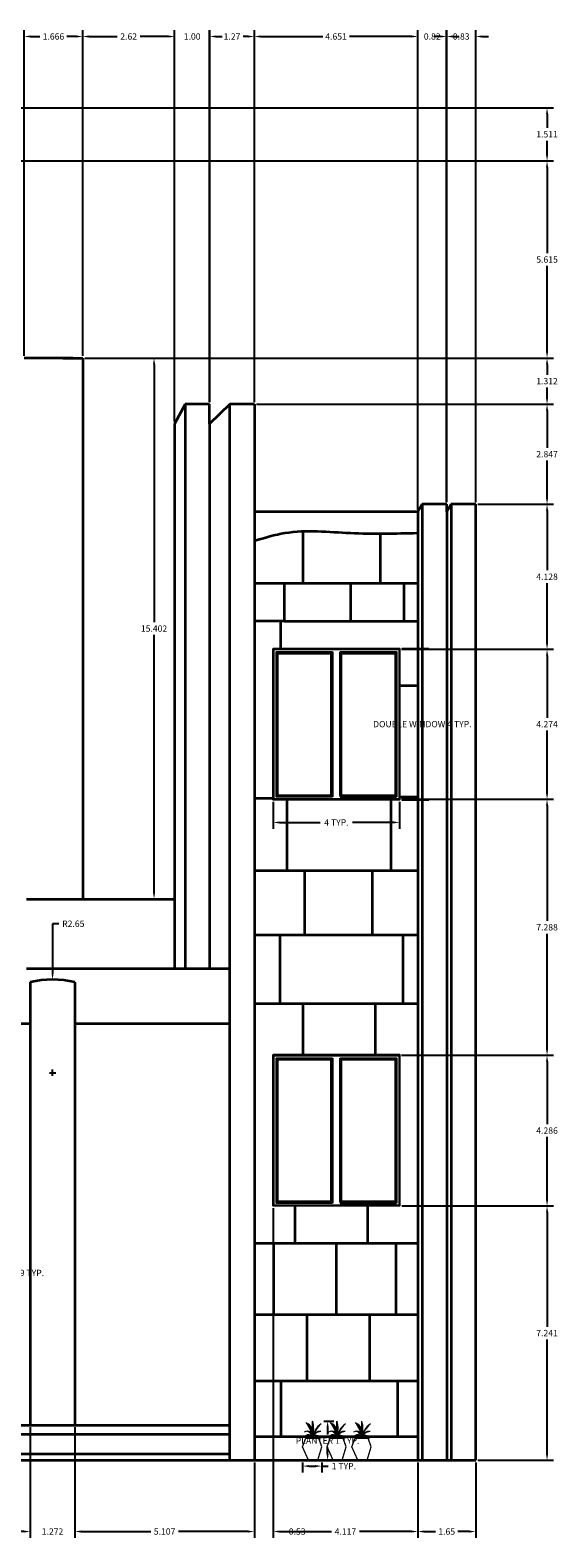
# Model space of a CAD drawing. Units: millimetres. Extents: x 2521.2 to 2565.9, y 755.2 to 798.1.
# Tile 3 of 3: x 2550.9 to 2565.9, y 755.2 to 798.1. Entities that reach past the tile are written whole.
import ezdxf

# ---------------------------------------------------------------- set-up
doc = ezdxf.new("R2010")
doc.units = ezdxf.units.MM
for name, color, linetype, lineweight in [('A-ANNO-DIMS', 2, 'Continuous', 18), ('A-ELEV', 7, 'Continuous', 35), ('A-GLAZ', 4, 'Continuous', 25), ('L-PLNT', 3, 'Continuous', 18)]:
    doc.layers.add(name, color=color, linetype=linetype, lineweight=lineweight)
doc.styles.get("Standard").update_dxf_attribs({"font": 'arial.ttf'})
doc.dimstyles.get("Standard").update_dxf_attribs({"dimtxt": 0.18, "dimasz": 0.18, "dimexe": 0.18, "dimexo": 0.0625, "dimgap": 0.09, "dimtad": 0, "dimtih": 1, "dimtoh": 1, "dimdec": 4, "dimzin": 0, "dimdsep": 46, "dimtxsty": 'Standard', "dimcen": 0.09, "dimadec": 0, "dimazin": 0, "dimtfac": 1, "dimtdec": 4, "dimtofl": 0, "dimtmove": 0, "dimatfit": 3, "dimfxl": 1, "dimtolj": 1, "dimtzin": 0, "dimarcsym": 0})

# ---------------------------------------------------------------- blocks, each defined once
blk = doc.blocks.new('WIN-DOUBLE')
for p, q in [((2559.456, 776.3), (2559.456, 780.343)), ((2559.491, 780.386), (2559.491, 776.258)), ((2559.716, 776.3), (2559.716, 780.386)), ((2559.756, 776.3), (2559.756, 780.343)), ((2559.716, 776.3), (2559.716, 776.258)), ((2559.716, 776.258), (2561.319, 776.258))]:
    blk.add_line(p, q)
for points in [[(2557.805, 780.483), (2561.406, 780.483), (2561.406, 776.176), (2557.805, 776.176)], [(2557.825, 780.462), (2561.393, 780.462), (2561.393, 776.189), (2557.825, 776.189)]]:
    blk.add_lwpolyline(points, close=True)
for points in [[(2559.491, 776.258), (2557.898, 776.258), (2557.898, 780.386), (2559.491, 780.386)], [(2559.456, 776.3), (2557.936, 776.3), (2557.936, 780.343), (2559.456, 780.343)], [(2559.716, 780.386), (2561.319, 780.386), (2561.319, 776.258)], [(2559.756, 780.343), (2561.276, 780.343), (2561.276, 776.3), (2559.756, 776.3)]]:
    blk.add_lwpolyline(points)
blk = doc.blocks.new('PLANTER')
for p, q in [((2558.646, 757.758), (2558.737, 758.005)), ((2558.817, 757.373), (2558.646, 757.758)), ((2558.737, 758.005), (2559.107, 758.005)), ((2559.08, 757.373), (2559.189, 757.758)), ((2559.189, 757.758), (2559.107, 758.005))]:
    blk.add_line(p, q)
for centre, radius, start, end in [((2558.164, 758.26), 0.796, 342.0282, 16.5628), ((2530.529, 758.527), 28.398, 358.9459, 359.9172), ((2558.772, 758.043), 0.155, 345.7039, 120.8927), ((2558.788, 757.931), 0.154, 28.8769, 113.7957), ((2558.504, 758.092), 0.427, 348.2161, 55.5831), ((2558.151, 757.944), 0.777, 5.6498, 40.0889), ((2558.161, 757.954), 0.763, 3.8104, 39.9888), ((2558.813, 757.985), 0.111, 10.1799, 119.9068), ((2558.697, 757.984), 0.226, 5.301, 71.0335), ((2558.66, 758.146), 0.293, 333.1798, 63.2065), ((2559.557, 757.89), 0.648, 126.493, 168.9551), ((2559.127, 757.986), 0.208, 79.6534, 172.2119), ((2559.023, 757.968), 0.112, 7.4318, 155.8017), ((2559.736, 757.784), 0.843, 132.0051, 164.8224), ((2559.176, 757.925), 0.266, 92.441, 162.4192), ((2559.033, 757.927), 0.136, 55.8779, 144.8755)]:
    blk.add_arc(centre, radius, start, end)
blk = doc.blocks.new('*D4')
at = {"layer": 'A-ANNO-DIMS', "color": 0, "lineweight": -2, "transparency": 16777216}
for p, q in [((2561.469, 780.483), (2562.232, 780.483)), ((2562.052, 780.303), (2562.052, 778.513)), ((2562.052, 776.356), (2562.052, 778.147)), ((2561.469, 776.176), (2562.232, 776.176))]:
    blk.add_line(p, q, dxfattribs=at)
at = {"layer": 'A-ANNO-DIMS', "color": 0, "transparency": 16777216}
for points in [[(2562.022, 780.303), (2562.082, 780.303), (2562.052, 780.483)], [(2562.022, 776.356), (2562.082, 776.356), (2562.052, 776.176)]]:
    blk.add_solid(points, dxfattribs=at)
at = {"layer": 'Defpoints', "color": 0, "transparency": 16777216}
for p in [(2561.406, 780.483), (2562.052, 780.483), (2561.406, 776.176)]:
    blk.add_point(p, dxfattribs=at)
at = {"layer": 'A-ANNO-DIMS', "color": 0, "transparency": 16777216, "insert": (2562.052, 778.33), "char_height": 0.18, "attachment_point": 5}
blk.add_mtext('\\A1;DOUBLE WINDOW 4 TYP.', dxfattribs=at)
blk = doc.blocks.new('*D5')
at = {"layer": 'A-ANNO-DIMS', "color": 0, "lineweight": -2, "transparency": 16777216}
for p, q in [((2557.805, 776.114), (2557.805, 775.35)), ((2561.406, 776.114), (2561.406, 775.35)), ((2557.985, 775.53), (2559.144, 775.53)), ((2561.226, 775.53), (2560.067, 775.53))]:
    blk.add_line(p, q, dxfattribs=at)
at = {"layer": 'A-ANNO-DIMS', "color": 0, "transparency": 16777216}
for points in [[(2557.985, 775.56), (2557.985, 775.5), (2557.805, 775.53)], [(2561.226, 775.56), (2561.226, 775.5), (2561.406, 775.53)]]:
    blk.add_solid(points, dxfattribs=at)
at = {"layer": 'Defpoints', "color": 0, "transparency": 16777216}
for p in [(2557.805, 776.176), (2561.406, 776.176), (2561.406, 775.53)]:
    blk.add_point(p, dxfattribs=at)
at = {"layer": 'A-ANNO-DIMS', "color": 0, "transparency": 16777216, "insert": (2559.606, 775.53), "char_height": 0.18, "attachment_point": 5}
blk.add_mtext('\\A1;4 TYP.', dxfattribs=at)
blk = doc.blocks.new('*D6')
at = {"layer": 'A-ANNO-DIMS', "color": 0, "lineweight": -2, "transparency": 16777216}
for p, q in [((2549.006, 767.037), (2550.423, 767.037)), ((2550.243, 766.857), (2550.243, 762.888)), ((2550.243, 758.553), (2550.243, 762.522)), ((2549.006, 758.373), (2550.423, 758.373))]:
    blk.add_line(p, q, dxfattribs=at)
at = {"layer": 'A-ANNO-DIMS', "color": 0, "transparency": 16777216}
for points in [[(2550.213, 766.857), (2550.273, 766.857), (2550.243, 767.037)], [(2550.213, 758.553), (2550.273, 758.553), (2550.243, 758.373)]]:
    blk.add_solid(points, dxfattribs=at)
at = {"layer": 'Defpoints', "color": 0, "transparency": 16777216}
for p in [(2548.944, 767.037), (2550.243, 767.037), (2548.944, 758.373)]:
    blk.add_point(p, dxfattribs=at)
at = {"layer": 'A-ANNO-DIMS', "color": 0, "transparency": 16777216, "insert": (2550.243, 762.705), "char_height": 0.18, "attachment_point": 5}
blk.add_mtext('\\A1;MAIN DOOR 9 TYP.', dxfattribs=at)
blk = doc.blocks.new('*D8')
at = {"layer": 'A-ANNO-DIMS', "color": 0, "lineweight": -2, "transparency": 16777216}
for p, q in [((2559.252, 758.486), (2559.536, 758.486)), ((2559.356, 758.306), (2559.356, 758.11)), ((2559.356, 757.553), (2559.356, 757.749)), ((2559.252, 757.373), (2559.536, 757.373))]:
    blk.add_line(p, q, dxfattribs=at)
at = {"layer": 'A-ANNO-DIMS', "color": 0, "transparency": 16777216}
for points in [[(2559.326, 758.306), (2559.386, 758.306), (2559.356, 758.486)], [(2559.326, 757.553), (2559.386, 757.553), (2559.356, 757.373)]]:
    blk.add_solid(points, dxfattribs=at)
at = {"layer": 'Defpoints', "color": 0, "transparency": 16777216}
for p in [(2559.189, 758.486), (2559.356, 758.486), (2559.189, 757.373)]:
    blk.add_point(p, dxfattribs=at)
at = {"layer": 'A-ANNO-DIMS', "color": 0, "transparency": 16777216, "insert": (2559.356, 757.93), "char_height": 0.18, "attachment_point": 5}
blk.add_mtext('\\A1;PLANTER 1 TYP.', dxfattribs=at)
blk = doc.blocks.new('*D9')
at = {"layer": 'A-ANNO-DIMS', "color": 0, "lineweight": -2, "transparency": 16777216}
for p, q in [((2558.646, 757.311), (2558.646, 757.026)), ((2558.826, 757.206), (2559.009, 757.206)), ((2559.189, 757.311), (2559.189, 757.026)), ((2559.189, 757.206), (2559.369, 757.206))]:
    blk.add_line(p, q, dxfattribs=at)
at = {"layer": 'A-ANNO-DIMS', "color": 0, "transparency": 16777216}
for points in [[(2558.826, 757.236), (2558.826, 757.176), (2558.646, 757.206)], [(2559.009, 757.236), (2559.009, 757.176), (2559.189, 757.206)]]:
    blk.add_solid(points, dxfattribs=at)
at = {"layer": 'Defpoints', "color": 0, "transparency": 16777216}
for p in [(2558.646, 757.373), (2559.189, 757.373), (2559.189, 757.206)]:
    blk.add_point(p, dxfattribs=at)
at = {"layer": 'A-ANNO-DIMS', "color": 0, "transparency": 16777216, "insert": (2559.819, 757.206), "char_height": 0.18, "attachment_point": 5}
blk.add_mtext('\\A1;1 TYP.', dxfattribs=at)
blk = doc.blocks.new('*D28')
at = {"layer": 'A-ANNO-DIMS', "color": 0, "lineweight": -2, "transparency": 16777216}
for p, q in [((2550.721, 788.812), (2550.721, 798.086)), ((2552.387, 788.812), (2552.387, 798.086)), ((2550.901, 797.906), (2551.169, 797.906)), ((2552.207, 797.906), (2551.939, 797.906))]:
    blk.add_line(p, q, dxfattribs=at)
at = {"layer": 'A-ANNO-DIMS', "color": 0, "transparency": 16777216}
for points in [[(2550.901, 797.936), (2550.901, 797.876), (2550.721, 797.906)], [(2552.207, 797.936), (2552.207, 797.876), (2552.387, 797.906)]]:
    blk.add_solid(points, dxfattribs=at)
at = {"layer": 'Defpoints', "color": 0, "transparency": 16777216}
for p in [(2552.387, 797.906), (2550.721, 788.75), (2552.387, 788.75)]:
    blk.add_point(p, dxfattribs=at)
at = {"layer": 'A-ANNO-DIMS', "color": 0, "transparency": 16777216, "insert": (2551.554, 797.906), "char_height": 0.18, "attachment_point": 5}
blk.add_mtext('\\A1;1.666', dxfattribs=at)
blk = doc.blocks.new('*D29')
at = {"layer": 'A-ANNO-DIMS', "color": 0, "lineweight": -2, "transparency": 16777216}
for p, q in [((2552.387, 788.812), (2552.387, 798.086)), ((2555.002, 786.941), (2555.002, 798.086)), ((2552.567, 797.906), (2553.37, 797.906)), ((2554.822, 797.906), (2554.019, 797.906))]:
    blk.add_line(p, q, dxfattribs=at)
at = {"layer": 'A-ANNO-DIMS', "color": 0, "transparency": 16777216}
for points in [[(2552.567, 797.936), (2552.567, 797.876), (2552.387, 797.906)], [(2554.822, 797.936), (2554.822, 797.876), (2555.002, 797.906)]]:
    blk.add_solid(points, dxfattribs=at)
at = {"layer": 'Defpoints', "color": 0, "transparency": 16777216}
for p in [(2555.002, 797.906), (2552.387, 788.75), (2555.002, 786.879)]:
    blk.add_point(p, dxfattribs=at)
at = {"layer": 'A-ANNO-DIMS', "color": 0, "transparency": 16777216, "insert": (2553.694, 797.906), "char_height": 0.18, "attachment_point": 5}
blk.add_mtext('\\A1;2.62', dxfattribs=at)
blk = doc.blocks.new('*D30')
at = {"layer": 'A-ANNO-DIMS', "color": 0, "lineweight": -2, "transparency": 16777216}
for p, q in [((2555.002138, 786.94116), (2555.002138, 798.086169)), ((2555.999594, 787.500222), (2555.999594, 798.086169)), ((2554.822138, 797.906169), (2554.642138, 797.906169)), ((2556.179594, 797.906169), (2556.359594, 797.906169))]:
    blk.add_line(p, q, dxfattribs=at)
at = {"layer": 'A-ANNO-DIMS', "color": 0, "transparency": 16777216}
for points in [[(2554.822138, 797.936169), (2554.822138, 797.876169), (2555.002138, 797.906169)], [(2556.179594, 797.936169), (2556.179594, 797.876169), (2555.999594, 797.906169)]]:
    blk.add_solid(points, dxfattribs=at)
at = {"layer": 'Defpoints', "color": 0, "transparency": 16777216}
for p in [(2555.999594, 797.906169), (2555.999594, 787.437722), (2555.002138, 786.87866)]:
    blk.add_point(p, dxfattribs=at)
at = {"layer": 'A-ANNO-DIMS', "color": 0, "transparency": 16777216, "insert": (2555.500866, 797.906169), "char_height": 0.18, "attachment_point": 5}
blk.add_mtext('\\A1;1.00', dxfattribs=at)
blk = doc.blocks.new('*D31')
at = {"layer": 'A-ANNO-DIMS', "color": 0, "lineweight": -2, "transparency": 16777216}
for p, q in [((2556, 787.5), (2556, 798.086)), ((2557.271, 787.5), (2557.271, 798.086)), ((2556.18, 797.906), (2556.32, 797.906)), ((2557.091, 797.906), (2556.951, 797.906))]:
    blk.add_line(p, q, dxfattribs=at)
at = {"layer": 'A-ANNO-DIMS', "color": 0, "transparency": 16777216}
for points in [[(2556.18, 797.936), (2556.18, 797.876), (2556, 797.906)], [(2557.091, 797.936), (2557.091, 797.876), (2557.271, 797.906)]]:
    blk.add_solid(points, dxfattribs=at)
at = {"layer": 'Defpoints', "color": 0, "transparency": 16777216}
for p in [(2557.271, 797.906), (2556, 787.438), (2557.271, 787.438)]:
    blk.add_point(p, dxfattribs=at)
at = {"layer": 'A-ANNO-DIMS', "color": 0, "transparency": 16777216, "insert": (2556.635, 797.906), "char_height": 0.18, "attachment_point": 5}
blk.add_mtext('\\A1;1.27', dxfattribs=at)
blk = doc.blocks.new('*D32')
at = {"layer": 'A-ANNO-DIMS', "color": 0, "lineweight": -2, "transparency": 16777216}
for p, q in [((2557.271, 787.5), (2557.271, 798.086)), ((2561.922, 784.436), (2561.922, 798.086)), ((2557.451, 797.906), (2559.217, 797.906)), ((2561.742, 797.906), (2559.976, 797.906))]:
    blk.add_line(p, q, dxfattribs=at)
at = {"layer": 'A-ANNO-DIMS', "color": 0, "transparency": 16777216}
for points in [[(2557.451, 797.936), (2557.451, 797.876), (2557.271, 797.906)], [(2561.742, 797.936), (2561.742, 797.876), (2561.922, 797.906)]]:
    blk.add_solid(points, dxfattribs=at)
at = {"layer": 'Defpoints', "color": 0, "transparency": 16777216}
for p in [(2561.922, 797.906), (2557.271, 787.438), (2561.922, 784.373)]:
    blk.add_point(p, dxfattribs=at)
at = {"layer": 'A-ANNO-DIMS', "color": 0, "transparency": 16777216, "insert": (2559.596, 797.906), "char_height": 0.18, "attachment_point": 5}
blk.add_mtext('\\A1;4.651', dxfattribs=at)
blk = doc.blocks.new('*D33')
at = {"layer": 'A-ANNO-DIMS', "color": 0, "lineweight": -2, "transparency": 16777216}
for p, q in [((2561.921891, 784.435917), (2561.921891, 798.086169)), ((2562.744309, 784.652956), (2562.744309, 798.086169)), ((2561.741891, 797.906169), (2561.561891, 797.906169)), ((2562.924309, 797.906169), (2563.104309, 797.906169))]:
    blk.add_line(p, q, dxfattribs=at)
at = {"layer": 'A-ANNO-DIMS', "color": 0, "transparency": 16777216}
for points in [[(2561.741891, 797.936169), (2561.741891, 797.876169), (2561.921891, 797.906169)], [(2562.924309, 797.936169), (2562.924309, 797.876169), (2562.744309, 797.906169)]]:
    blk.add_solid(points, dxfattribs=at)
at = {"layer": 'Defpoints', "color": 0, "transparency": 16777216}
for p in [(2562.744309, 797.906169), (2561.921891, 784.373417), (2562.744309, 784.590456)]:
    blk.add_point(p, dxfattribs=at)
at = {"layer": 'A-ANNO-DIMS', "color": 0, "transparency": 16777216, "insert": (2562.3331, 797.906169), "char_height": 0.18, "attachment_point": 5}
blk.add_mtext('\\A1;0.82', dxfattribs=at)
blk = doc.blocks.new('*D34')
at = {"layer": 'A-ANNO-DIMS', "color": 0, "lineweight": -2, "transparency": 16777216}
for p, q in [((2562.744, 784.653), (2562.744, 798.086)), ((2563.571, 784.653), (2563.571, 798.086)), ((2562.564, 797.906), (2562.384, 797.906)), ((2563.751, 797.906), (2563.931, 797.906))]:
    blk.add_line(p, q, dxfattribs=at)
at = {"layer": 'A-ANNO-DIMS', "color": 0, "transparency": 16777216}
for points in [[(2562.564, 797.936), (2562.564, 797.876), (2562.744, 797.906)], [(2563.751, 797.936), (2563.751, 797.876), (2563.571, 797.906)]]:
    blk.add_solid(points, dxfattribs=at)
at = {"layer": 'Defpoints', "color": 0, "transparency": 16777216}
for p in [(2563.571, 797.906), (2562.744, 784.59), (2563.571, 784.59)]:
    blk.add_point(p, dxfattribs=at)
at = {"layer": 'A-ANNO-DIMS', "color": 0, "transparency": 16777216, "insert": (2563.158, 797.906), "char_height": 0.18, "attachment_point": 5}
blk.add_mtext('\\A1;0.83', dxfattribs=at)
blk = doc.blocks.new('*D46')
at = {"layer": 'A-ANNO-DIMS', "color": 0, "lineweight": -2, "transparency": 16777216}
for p, q in [((2550.891519, 758.310917), (2550.891519, 755.163417)), ((2552.163561, 758.310917), (2552.163561, 755.163417)), ((2550.711519, 755.343417), (2550.531519, 755.343417)), ((2552.343561, 755.343417), (2552.523561, 755.343417))]:
    blk.add_line(p, q, dxfattribs=at)
at = {"layer": 'A-ANNO-DIMS', "color": 0, "transparency": 16777216}
for points in [[(2550.711519, 755.373417), (2550.711519, 755.313417), (2550.891519, 755.343417)], [(2552.343561, 755.373417), (2552.343561, 755.313417), (2552.163561, 755.343417)]]:
    blk.add_solid(points, dxfattribs=at)
at = {"layer": 'Defpoints', "color": 0, "transparency": 16777216}
for p in [(2550.891519, 758.373417), (2552.163561, 758.373417), (2552.163561, 755.343417)]:
    blk.add_point(p, dxfattribs=at)
at = {"layer": 'A-ANNO-DIMS', "color": 0, "transparency": 16777216, "insert": (2551.52754, 755.343417), "char_height": 0.18, "attachment_point": 5}
blk.add_mtext('\\A1;1.272', dxfattribs=at)
blk = doc.blocks.new('*D47')
at = {"layer": 'A-ANNO-DIMS', "color": 0, "lineweight": -2, "transparency": 16777216}
for p, q in [((2552.164, 758.311), (2552.164, 755.163)), ((2557.271, 757.311), (2557.271, 755.163)), ((2552.344, 755.343), (2554.324, 755.343)), ((2557.091, 755.343), (2555.111, 755.343))]:
    blk.add_line(p, q, dxfattribs=at)
at = {"layer": 'A-ANNO-DIMS', "color": 0, "transparency": 16777216}
for points in [[(2552.344, 755.373), (2552.344, 755.313), (2552.164, 755.343)], [(2557.091, 755.373), (2557.091, 755.313), (2557.271, 755.343)]]:
    blk.add_solid(points, dxfattribs=at)
at = {"layer": 'Defpoints', "color": 0, "transparency": 16777216}
for p in [(2552.164, 758.373), (2557.271, 757.373), (2557.271, 755.343)]:
    blk.add_point(p, dxfattribs=at)
at = {"layer": 'A-ANNO-DIMS', "color": 0, "transparency": 16777216, "insert": (2554.717, 755.343), "char_height": 0.18, "attachment_point": 5}
blk.add_mtext('\\A1;5.107', dxfattribs=at)
blk = doc.blocks.new('*D48')
at = {"layer": 'A-ANNO-DIMS', "color": 0, "lineweight": -2, "transparency": 16777216}
for p, q in [((2557.805, 764.552), (2557.805, 755.163)), ((2557.271, 757.311), (2557.271, 755.163)), ((2557.091, 755.343), (2556.911, 755.343)), ((2557.985, 755.343), (2558.165, 755.343))]:
    blk.add_line(p, q, dxfattribs=at)
at = {"layer": 'A-ANNO-DIMS', "color": 0, "transparency": 16777216}
for points in [[(2557.091, 755.373), (2557.091, 755.313), (2557.271, 755.343)], [(2557.985, 755.373), (2557.985, 755.313), (2557.805, 755.343)]]:
    blk.add_solid(points, dxfattribs=at)
at = {"layer": 'Defpoints', "color": 0, "transparency": 16777216}
for p in [(2557.805, 764.614), (2557.271, 757.373), (2557.805, 755.343)]:
    blk.add_point(p, dxfattribs=at)
at = {"layer": 'A-ANNO-DIMS', "color": 0, "transparency": 16777216, "insert": (2558.489, 755.343), "char_height": 0.18, "attachment_point": 5}
blk.add_mtext('\\A1;0.53', dxfattribs=at)
blk = doc.blocks.new('*D49')
at = {"layer": 'A-ANNO-DIMS', "color": 0, "lineweight": -2, "transparency": 16777216}
for p, q in [((2557.805, 764.552), (2557.805, 755.163)), ((2561.922, 757.311), (2561.922, 755.163)), ((2557.985, 755.343), (2559.466, 755.343)), ((2561.742, 755.343), (2560.261, 755.343))]:
    blk.add_line(p, q, dxfattribs=at)
at = {"layer": 'A-ANNO-DIMS', "color": 0, "transparency": 16777216}
for points in [[(2557.985, 755.373), (2557.985, 755.313), (2557.805, 755.343)], [(2561.742, 755.373), (2561.742, 755.313), (2561.922, 755.343)]]:
    blk.add_solid(points, dxfattribs=at)
at = {"layer": 'Defpoints', "color": 0, "transparency": 16777216}
for p in [(2557.805, 764.614), (2561.922, 757.373), (2561.922, 755.343)]:
    blk.add_point(p, dxfattribs=at)
at = {"layer": 'A-ANNO-DIMS', "color": 0, "transparency": 16777216, "insert": (2559.863, 755.343), "char_height": 0.18, "attachment_point": 5}
blk.add_mtext('\\A1;4.117', dxfattribs=at)
blk = doc.blocks.new('*D50')
at = {"layer": 'A-ANNO-DIMS', "color": 0, "lineweight": -2, "transparency": 16777216}
for p, q in [((2561.922, 757.311), (2561.922, 755.163)), ((2563.571, 757.311), (2563.571, 755.163)), ((2562.102, 755.343), (2562.43, 755.343)), ((2563.391, 755.343), (2563.062, 755.343))]:
    blk.add_line(p, q, dxfattribs=at)
at = {"layer": 'A-ANNO-DIMS', "color": 0, "transparency": 16777216}
for points in [[(2562.102, 755.373), (2562.102, 755.313), (2561.922, 755.343)], [(2563.391, 755.373), (2563.391, 755.313), (2563.571, 755.343)]]:
    blk.add_solid(points, dxfattribs=at)
at = {"layer": 'Defpoints', "color": 0, "transparency": 16777216}
for p in [(2561.922, 757.373), (2563.571, 757.373), (2563.571, 755.343)]:
    blk.add_point(p, dxfattribs=at)
at = {"layer": 'A-ANNO-DIMS', "color": 0, "transparency": 16777216, "insert": (2562.746, 755.343), "char_height": 0.18, "attachment_point": 5}
blk.add_mtext('\\A1;1.65', dxfattribs=at)
blk = doc.blocks.new('*D51')
at = {"layer": 'A-ANNO-DIMS', "color": 0, "lineweight": -2, "transparency": 16777216}
for p, q in [((2561.469, 764.614), (2565.781, 764.614)), ((2565.601, 764.434), (2565.601, 761.174)), ((2565.601, 757.553), (2565.601, 760.814)), ((2563.634, 757.373), (2565.781, 757.373))]:
    blk.add_line(p, q, dxfattribs=at)
at = {"layer": 'A-ANNO-DIMS', "color": 0, "transparency": 16777216}
for points in [[(2565.571, 764.434), (2565.631, 764.434), (2565.601, 764.614)], [(2565.571, 757.553), (2565.631, 757.553), (2565.601, 757.373)]]:
    blk.add_solid(points, dxfattribs=at)
at = {"layer": 'Defpoints', "color": 0, "transparency": 16777216}
for p in [(2561.406, 764.614), (2565.601, 764.614), (2563.571, 757.373)]:
    blk.add_point(p, dxfattribs=at)
at = {"layer": 'A-ANNO-DIMS', "color": 0, "transparency": 16777216, "insert": (2565.601, 760.994), "char_height": 0.18, "attachment_point": 5}
blk.add_mtext('\\A1;7.241', dxfattribs=at)
blk = doc.blocks.new('*D52')
at = {"layer": 'A-ANNO-DIMS', "color": 0, "lineweight": -2, "transparency": 16777216}
for p, q in [((2561.455, 768.901), (2565.781, 768.901)), ((2565.601, 768.721), (2565.601, 766.939)), ((2565.601, 764.794), (2565.601, 766.576)), ((2561.469, 764.614), (2565.781, 764.614))]:
    blk.add_line(p, q, dxfattribs=at)
at = {"layer": 'A-ANNO-DIMS', "color": 0, "transparency": 16777216}
for points in [[(2565.571, 768.721), (2565.631, 768.721), (2565.601, 768.901)], [(2565.571, 764.794), (2565.631, 764.794), (2565.601, 764.614)]]:
    blk.add_solid(points, dxfattribs=at)
at = {"layer": 'Defpoints', "color": 0, "transparency": 16777216}
for p in [(2561.393, 768.901), (2565.601, 768.901), (2561.406, 764.614)]:
    blk.add_point(p, dxfattribs=at)
at = {"layer": 'A-ANNO-DIMS', "color": 0, "transparency": 16777216, "insert": (2565.601, 766.758), "char_height": 0.18, "attachment_point": 5}
blk.add_mtext('\\A1;4.286', dxfattribs=at)
blk = doc.blocks.new('*D53')
at = {"layer": 'A-ANNO-DIMS', "color": 0, "lineweight": -2, "transparency": 16777216}
for p, q in [((2561.455, 776.189), (2565.781, 776.189)), ((2565.601, 776.009), (2565.601, 772.726)), ((2565.601, 769.081), (2565.601, 772.363)), ((2561.455, 768.901), (2565.781, 768.901))]:
    blk.add_line(p, q, dxfattribs=at)
at = {"layer": 'A-ANNO-DIMS', "color": 0, "transparency": 16777216}
for points in [[(2565.571, 776.009), (2565.631, 776.009), (2565.601, 776.189)], [(2565.571, 769.081), (2565.631, 769.081), (2565.601, 768.901)]]:
    blk.add_solid(points, dxfattribs=at)
at = {"layer": 'Defpoints', "color": 0, "transparency": 16777216}
for p in [(2561.393, 776.189), (2565.601, 776.189), (2561.393, 768.901)]:
    blk.add_point(p, dxfattribs=at)
at = {"layer": 'A-ANNO-DIMS', "color": 0, "transparency": 16777216, "insert": (2565.601, 772.545), "char_height": 0.18, "attachment_point": 5}
blk.add_mtext('\\A1;7.288', dxfattribs=at)
blk = doc.blocks.new('*D54')
at = {"layer": 'A-ANNO-DIMS', "color": 0, "lineweight": -2, "transparency": 16777216}
for p, q in [((2561.455, 780.462), (2565.781, 780.462)), ((2565.601, 780.282), (2565.601, 778.506)), ((2565.601, 776.369), (2565.601, 778.145)), ((2561.455, 776.189), (2565.781, 776.189))]:
    blk.add_line(p, q, dxfattribs=at)
at = {"layer": 'A-ANNO-DIMS', "color": 0, "transparency": 16777216}
for points in [[(2565.571, 780.282), (2565.631, 780.282), (2565.601, 780.462)], [(2565.571, 776.369), (2565.631, 776.369), (2565.601, 776.189)]]:
    blk.add_solid(points, dxfattribs=at)
at = {"layer": 'Defpoints', "color": 0, "transparency": 16777216}
for p in [(2561.393, 780.462), (2565.601, 780.462), (2561.393, 776.189)]:
    blk.add_point(p, dxfattribs=at)
at = {"layer": 'A-ANNO-DIMS', "color": 0, "transparency": 16777216, "insert": (2565.601, 778.326), "char_height": 0.18, "attachment_point": 5}
blk.add_mtext('\\A1;4.274', dxfattribs=at)
blk = doc.blocks.new('*D55')
at = {"layer": 'A-ANNO-DIMS', "color": 0, "lineweight": -2, "transparency": 16777216}
for p, q in [((2563.634, 784.59), (2565.781, 784.59)), ((2565.601, 784.41), (2565.601, 782.708)), ((2565.601, 780.642), (2565.601, 782.345)), ((2561.455, 780.462), (2565.781, 780.462))]:
    blk.add_line(p, q, dxfattribs=at)
at = {"layer": 'A-ANNO-DIMS', "color": 0, "transparency": 16777216}
for points in [[(2565.571, 784.41), (2565.631, 784.41), (2565.601, 784.59)], [(2565.571, 780.642), (2565.631, 780.642), (2565.601, 780.462)]]:
    blk.add_solid(points, dxfattribs=at)
at = {"layer": 'Defpoints', "color": 0, "transparency": 16777216}
for p in [(2563.571, 784.59), (2565.601, 784.59), (2561.393, 780.462)]:
    blk.add_point(p, dxfattribs=at)
at = {"layer": 'A-ANNO-DIMS', "color": 0, "transparency": 16777216, "insert": (2565.601, 782.526), "char_height": 0.18, "attachment_point": 5}
blk.add_mtext('\\A1;4.128', dxfattribs=at)
blk = doc.blocks.new('*D56')
at = {"layer": 'A-ANNO-DIMS', "color": 0, "lineweight": -2, "transparency": 16777216}
for p, q in [((2557.334, 787.438), (2565.781, 787.438)), ((2565.601, 787.258), (2565.601, 786.196)), ((2565.601, 784.77), (2565.601, 785.832)), ((2563.634, 784.59), (2565.781, 784.59))]:
    blk.add_line(p, q, dxfattribs=at)
at = {"layer": 'A-ANNO-DIMS', "color": 0, "transparency": 16777216}
for points in [[(2565.571, 787.258), (2565.631, 787.258), (2565.601, 787.438)], [(2565.571, 784.77), (2565.631, 784.77), (2565.601, 784.59)]]:
    blk.add_solid(points, dxfattribs=at)
at = {"layer": 'Defpoints', "color": 0, "transparency": 16777216}
for p in [(2557.271, 787.438), (2565.601, 787.438), (2563.571, 784.59)]:
    blk.add_point(p, dxfattribs=at)
at = {"layer": 'A-ANNO-DIMS', "color": 0, "transparency": 16777216, "insert": (2565.601, 786.014), "char_height": 0.18, "attachment_point": 5}
blk.add_mtext('\\A1;2.847', dxfattribs=at)
blk = doc.blocks.new('*D57')
at = {"layer": 'A-ANNO-DIMS', "color": 0, "lineweight": -2, "transparency": 16777216}
for p, q in [((2552.449, 788.75), (2565.781, 788.75)), ((2565.601, 788.57), (2565.601, 788.276)), ((2565.601, 787.618), (2565.601, 787.912)), ((2557.334, 787.438), (2565.781, 787.438))]:
    blk.add_line(p, q, dxfattribs=at)
at = {"layer": 'A-ANNO-DIMS', "color": 0, "transparency": 16777216}
for points in [[(2565.571, 788.57), (2565.631, 788.57), (2565.601, 788.75)], [(2565.571, 787.618), (2565.631, 787.618), (2565.601, 787.438)]]:
    blk.add_solid(points, dxfattribs=at)
at = {"layer": 'Defpoints', "color": 0, "transparency": 16777216}
for p in [(2552.387, 788.75), (2565.601, 788.75), (2557.271, 787.438)]:
    blk.add_point(p, dxfattribs=at)
at = {"layer": 'A-ANNO-DIMS', "color": 0, "transparency": 16777216, "insert": (2565.601, 788.094), "char_height": 0.18, "attachment_point": 5}
blk.add_mtext('\\A1;1.312', dxfattribs=at)
blk = doc.blocks.new('*D58')
at = {"layer": 'A-ANNO-DIMS', "color": 0, "lineweight": -2, "transparency": 16777216}
for p, q in [((2549.109, 794.365), (2565.781, 794.365)), ((2565.601, 794.185), (2565.601, 791.739)), ((2565.601, 788.93), (2565.601, 791.376)), ((2552.449, 788.75), (2565.781, 788.75))]:
    blk.add_line(p, q, dxfattribs=at)
at = {"layer": 'A-ANNO-DIMS', "color": 0, "transparency": 16777216}
for points in [[(2565.571, 794.185), (2565.631, 794.185), (2565.601, 794.365)], [(2565.571, 788.93), (2565.631, 788.93), (2565.601, 788.75)]]:
    blk.add_solid(points, dxfattribs=at)
at = {"layer": 'Defpoints', "color": 0, "transparency": 16777216}
for p in [(2549.046, 794.365), (2565.601, 794.365), (2552.387, 788.75)]:
    blk.add_point(p, dxfattribs=at)
at = {"layer": 'A-ANNO-DIMS', "color": 0, "transparency": 16777216, "insert": (2565.601, 791.557), "char_height": 0.18, "attachment_point": 5}
blk.add_mtext('\\A1;5.615', dxfattribs=at)
blk = doc.blocks.new('*D59')
at = {"layer": 'A-ANNO-DIMS', "color": 0, "lineweight": -2, "transparency": 16777216}
for p, q in [((2549.109, 795.876), (2565.781, 795.876)), ((2565.601, 795.696), (2565.601, 795.303)), ((2565.601, 794.545), (2565.601, 794.939)), ((2549.109, 794.365), (2565.781, 794.365))]:
    blk.add_line(p, q, dxfattribs=at)
at = {"layer": 'A-ANNO-DIMS', "color": 0, "transparency": 16777216}
for points in [[(2565.571, 795.696), (2565.631, 795.696), (2565.601, 795.876)], [(2565.571, 794.545), (2565.631, 794.545), (2565.601, 794.365)]]:
    blk.add_solid(points, dxfattribs=at)
at = {"layer": 'Defpoints', "color": 0, "transparency": 16777216}
for p in [(2549.046, 795.876), (2565.601, 795.876), (2549.046, 794.365)]:
    blk.add_point(p, dxfattribs=at)
at = {"layer": 'A-ANNO-DIMS', "color": 0, "transparency": 16777216, "insert": (2565.601, 795.121), "char_height": 0.18, "attachment_point": 5}
blk.add_mtext('\\A1;1.511', dxfattribs=at)
blk = doc.blocks.new('*D66')
at = {"layer": 'A-ANNO-DIMS', "color": 0, "lineweight": -2, "transparency": 16777216}
for p, q in [((2552.449, 788.75), (2554.597, 788.75)), ((2554.417, 788.57), (2554.417, 781.231)), ((2554.417, 773.528), (2554.417, 780.867)), ((2552.449, 773.348), (2554.597, 773.348))]:
    blk.add_line(p, q, dxfattribs=at)
at = {"layer": 'A-ANNO-DIMS', "color": 0, "transparency": 16777216}
for points in [[(2554.387, 788.57), (2554.447, 788.57), (2554.417, 788.75)], [(2554.387, 773.528), (2554.447, 773.528), (2554.417, 773.348)]]:
    blk.add_solid(points, dxfattribs=at)
at = {"layer": 'Defpoints', "color": 0, "transparency": 16777216}
for p in [(2552.387, 788.75), (2552.387, 773.348), (2554.417, 773.348)]:
    blk.add_point(p, dxfattribs=at)
at = {"layer": 'A-ANNO-DIMS', "color": 0, "transparency": 16777216, "insert": (2554.417, 781.049), "char_height": 0.18, "attachment_point": 5}
blk.add_mtext('\\A1;15.402', dxfattribs=at)
blk = doc.blocks.new('*D67')
at = {"layer": 'A-ANNO-DIMS', "color": 0, "lineweight": -2, "transparency": 16777216}
for p, q in [((2551.708, 772.647), (2551.528, 772.647)), ((2551.528, 772.647), (2551.528, 771.237)), ((2551.438, 768.406), (2551.618, 768.406)), ((2551.528, 768.316), (2551.528, 768.496))]:
    blk.add_line(p, q, dxfattribs=at)
at = {"layer": 'A-ANNO-DIMS', "color": 0, "transparency": 16777216}
blk.add_solid([(2551.498, 771.237), (2551.558, 771.237), (2551.528, 771.057)], dxfattribs=at)
at = {"layer": 'Defpoints', "color": 0, "transparency": 16777216}
for p in [(2551.528, 771.057), (2551.528, 768.406)]:
    blk.add_point(p, dxfattribs=at)
at = {"layer": 'A-ANNO-DIMS', "color": 0, "transparency": 16777216, "insert": (2552.119, 772.647), "char_height": 0.18, "attachment_point": 5}
blk.add_mtext('\\A1;R2.65', dxfattribs=at)

msp = doc.modelspace()

# ---------------------------------------------------------------- linework, layer by layer
at = {"layer": 'A-ELEV'}
for p, q in [((2552.1043, 788.7497), (2550.7207, 788.7497)), ((2551.8217, 788.7497), (2552.3868, 788.7497)), ((2552.3868, 788.7497), (2552.3868, 773.3478)), ((2555.2996, 787.4377), (2555.0021, 786.8787)), ((2555.9996, 787.4377), (2555.2996, 787.4377)), ((2555.2996, 787.4377), (2555.2996, 771.3734)), ((2556.5711, 787.4377), (2555.9996, 786.8787)), ((2555.9996, 786.8787), (2555.9996, 787.4377)), ((2556.5711, 758.3734), (2556.5711, 787.4377)), ((2557.2711, 787.4377), (2556.5711, 787.4377)), ((2557.2711, 787.4377), (2557.2711, 757.3734)), ((2555.0021, 786.8787), (2555.0021, 771.3734)), ((2555.9996, 786.8787), (2555.9996, 773.8787)), ((2561.9219, 784.3734), (2557.2711, 784.3734)), ((2562.0443, 784.5905), (2561.9219, 784.3734)), ((2561.9219, 784.3734), (2561.9219, 757.3734)), ((2562.7443, 784.5905), (2562.0443, 784.5905)), ((2562.0443, 784.5905), (2562.0443, 757.3734)), ((2562.8711, 784.5905), (2562.7443, 784.3734)), ((2562.7443, 784.3734), (2562.7443, 784.5905)), ((2562.7443, 784.3734), (2562.7443, 757.3734)), ((2563.5711, 784.5905), (2562.8711, 784.5905)), ((2562.8711, 784.5905), (2562.8711, 757.3734)), ((2563.5711, 784.3734), (2563.5711, 784.5905)), ((2563.5711, 782.3734), (2563.5711, 784.3734)), ((2558.6553, 783.8203), (2558.6553, 782.3436)), ((2560.8562, 783.7562), (2560.8562, 782.3436)), ((2557.2711, 782.3436), (2561.9219, 782.3436)), ((2558.1243, 782.3436), (2558.1243, 781.2597)), ((2560.0102, 782.3436), (2560.0102, 781.2597)), ((2561.5259, 782.3436), (2561.5259, 781.2597)), ((2563.5711, 779.3734), (2563.5711, 782.3734)), ((2558.1243, 781.2597), (2557.2711, 781.2597)), ((2558.0167, 781.2597), (2558.0167, 780.4832)), ((2558.1243, 781.2597), (2561.9219, 781.2597)), ((2561.4064, 779.4334), (2561.9219, 779.4334)), ((2563.5711, 769.3734), (2563.5711, 779.3734)), ((2557.8048, 776.2091), (2557.2711, 776.2091)), ((2558.1982, 776.1764), (2558.1982, 774.1657)), ((2561.1568, 776.1764), (2561.1568, 774.1657)), ((2561.4064, 776.2608), (2561.9219, 776.2608)), ((2557.2711, 774.1657), (2561.9219, 774.1657)), ((2558.6957, 774.1657), (2558.6957, 772.3299)), ((2560.625, 774.1657), (2560.625, 772.3299)), ((2555.9996, 773.8787), (2555.9996, 771.3734)), ((2550.7859, 773.3478), (2555.0021, 773.3478)), ((2557.2711, 772.3299), (2561.9219, 772.3299)), ((2557.9975, 772.3299), (2557.9975, 770.3717)), ((2561.4963, 772.3299), (2561.4963, 770.3717)), ((2550.7859, 771.3734), (2556.5711, 771.3734)), ((2550.8915, 770.9792), (2550.8915, 758.3734)), ((2552.1636, 770.9792), (2552.1636, 758.3734)), ((2557.2711, 770.3717), (2561.9219, 770.3717)), ((2558.6538, 770.3717), (2558.6538, 768.9213)), ((2560.7095, 770.3717), (2560.7095, 768.9213)), ((2535.8411, 769.807), (2550.8915, 769.807)), ((2552.1636, 769.807), (2556.5711, 769.807)), ((2563.5711, 768.3734), (2563.5711, 769.3734)), ((2563.5711, 758.3734), (2563.5711, 768.3734)), ((2558.4262, 764.6145), (2558.4262, 763.5564)), ((2560.4906, 764.6145), (2560.4906, 763.5564)), ((2557.2711, 763.5564), (2561.9219, 763.5564)), ((2557.8186, 763.5564), (2557.8186, 761.52)), ((2559.5965, 763.5564), (2559.5965, 761.52)), ((2561.2965, 763.5564), (2561.2965, 761.52)), ((2557.2711, 761.52), (2561.9219, 761.52)), ((2558.7692, 761.52), (2558.7692, 759.6302)), ((2560.5513, 761.52), (2560.5513, 759.6302)), ((2557.2711, 759.6302), (2561.9219, 759.6302)), ((2558.0272, 759.6302), (2558.0272, 758.0459)), ((2561.3484, 759.6302), (2561.3484, 758.0459)), ((2539.7823, 758.3734), (2556.5711, 758.3734)), ((2539.7823, 758.1133), (2556.5711, 758.1133)), ((2556.5711, 757.3734), (2556.5711, 758.3734)), ((2557.2711, 758.0459), (2561.9219, 758.0459)), ((2563.5711, 757.3734), (2563.5711, 758.3734)), ((2523.5711, 757.3734), (2563.5711, 757.3734)), ((2539.7823, 757.5506), (2556.5711, 757.5506))]:
    msp.add_line(p, q, dxfattribs=at)
msp.add_arc((2551.5275, 768.4063), 2.6503, 76.11477, 103.88523, dxfattribs=at)
msp.add_open_spline([(2557.2711, 783.5497), (2557.5623, 783.6375), (2558.4489, 783.9048), (2560.0304, 783.7296), (2561.2842, 783.7585), (2561.9219, 783.7731)], degree=3, knots=[0, 0, 0, 0, 0.9066182, 2.7602692, 4.6787923, 4.6787923, 4.6787923, 4.6787923], dxfattribs=at)

# ---------------------------------------------------------------- block references
at = {"layer": 'A-GLAZ'}
for p in [(0, 0), (0, -11.562)]:
    msp.add_blockref('WIN-DOUBLE', p, dxfattribs=at)
at = {"layer": 'L-PLNT'}
for p in [(0, 0), (0.6937, 0), (1.4022, 0)]:
    msp.add_blockref('PLANTER', p, dxfattribs=at)

# ---------------------------------------------------------------- dimensions: what is measured, and where the dimension line sits
at = {"layer": 'A-ANNO-DIMS'}
for base, p1, p2, override, picture, middle in [((2552.3868, 797.9062), (2550.7207, 788.7497), (2552.3868, 788.7497), {"dimdec": 3, "dimlfac": 1, "dimrnd": 0, "dimzin": 0, "dimdsep": 46, "dimlunit": 2}, '*D28', (2551.5538, 797.9062)), ((2555.0021, 797.9062), (2552.3868, 788.7497), (2555.0021, 786.8787), {"dimdec": 2, "dimlfac": 1, "dimrnd": 0, "dimzin": 0, "dimdsep": 46, "dimlunit": 2}, '*D29', (2553.6945, 797.9062)), ((2555.9996, 797.9062), (2555.0021, 786.8787), (2555.9996, 787.4377), {"dimdec": 2, "dimlfac": 1, "dimrnd": 0, "dimzin": 0, "dimdsep": 46, "dimlunit": 2}, '*D30', (2555.5009, 797.9062)), ((2557.2711, 797.9062), (2555.9996, 787.4377), (2557.2711, 787.4377), {"dimdec": 2, "dimlfac": 1, "dimrnd": 0, "dimzin": 0, "dimdsep": 46, "dimlunit": 2}, '*D31', (2556.6353, 797.9062)), ((2561.9219, 797.9062), (2557.2711, 787.4377), (2561.9219, 784.3734), {"dimdec": 3, "dimlfac": 1, "dimrnd": 0, "dimzin": 0, "dimdsep": 46, "dimlunit": 2}, '*D32', (2559.5965, 797.9062)), ((2562.7443, 797.9062), (2561.9219, 784.3734), (2562.7443, 784.5905), {"dimdec": 2, "dimlfac": 1, "dimrnd": 0, "dimzin": 0, "dimdsep": 46, "dimlunit": 2}, '*D33', (2562.3331, 797.9062)), ((2563.5711, 797.9062), (2562.7443, 784.5905), (2563.5711, 784.5905), {"dimdec": 2, "dimlfac": 1, "dimrnd": 0, "dimzin": 0, "dimdsep": 46, "dimlunit": 2}, '*D34', (2563.1577, 797.9062)), ((2557.8048, 755.3434), (2557.2711, 757.3734), (2557.8048, 764.6145), {"dimdec": 2, "dimlfac": 1, "dimrnd": 0, "dimzin": 0, "dimdsep": 46, "dimlunit": 2}, '*D48', (2558.4886, 755.3434)), ((2561.9219, 755.3434), (2557.8048, 764.6145), (2561.9219, 757.3734), {"dimdec": 3, "dimlfac": 1, "dimrnd": 0, "dimzin": 0, "dimdsep": 46, "dimlunit": 2}, '*D49', (2559.8634, 755.3434)), ((2552.1636, 755.3434), (2550.8915, 758.3734), (2552.1636, 758.3734), {"dimdec": 3, "dimlfac": 1, "dimrnd": 0, "dimzin": 0, "dimdsep": 46, "dimlunit": 2}, '*D46', (2551.5275, 755.3434)), ((2557.271056, 755.343417), (2552.163561, 758.373417), (2557.271056, 757.373417), {"dimdec": 3, "dimlfac": 1, "dimrnd": 0, "dimzin": 0, "dimdsep": 46, "dimlunit": 2}, '*D47', (2554.717308, 755.343417)), ((2563.5711, 755.3434), (2561.9219, 757.3734), (2563.5711, 757.3734), {"dimdec": 2, "dimlfac": 1, "dimrnd": 0, "dimzin": 0, "dimdsep": 46, "dimlunit": 2}, '*D50', (2562.7465, 755.3434))]:
    dim = msp.add_linear_dim(base=base, p1=p1, p2=p2, dimstyle='Standard', override=override, dxfattribs=at)
    dim.commit()
    dim.dimension.update_dxf_attribs({"geometry": picture, "text_midpoint": middle})
for base, p1, p2, angle, picture, middle in [((2565.6011, 795.8762), (2549.0464, 794.3652), (2549.0464, 795.8762), 90, '*D59', (2565.6011, 795.1207)), ((2565.60106, 794.36515), (2552.38684, 788.7497), (2549.04639, 794.36515), 90, '*D58', (2565.60106, 791.55743)), ((2565.6011, 788.7497), (2557.2711, 787.4377), (2552.3868, 788.7497), 90, '*D57', (2565.6011, 788.0937)), ((2554.4168, 773.3478), (2552.3868, 788.7497), (2552.3868, 773.3478), 270, '*D66', (2554.4168, 781.0487)), ((2565.6011, 787.4377), (2563.5711, 784.5905), (2557.2711, 787.4377), 90, '*D56', (2565.6011, 786.0141)), ((2565.6011, 784.5905), (2561.3928, 780.4625), (2563.5711, 784.5905), 90, '*D55', (2565.6011, 782.5265)), ((2565.6011, 780.4625), (2561.3928, 776.1886), (2561.3928, 780.4625), 90, '*D54', (2565.6011, 778.3256)), ((2565.6011, 776.1886), (2561.3928, 768.9005), (2561.3928, 776.1886), 90, '*D53', (2565.6011, 772.5446)), ((2565.6011, 768.9005), (2561.4064, 764.6145), (2561.3928, 768.9005), 90, '*D52', (2565.6011, 766.7575)), ((2565.6011, 764.6145), (2563.5711, 757.3734), (2561.4064, 764.6145), 90, '*D51', (2565.6011, 760.9939))]:
    dim = msp.add_linear_dim(base=base, p1=p1, p2=p2, angle=angle, dimstyle='Standard', override={"dimdec": 3, "dimlfac": 1, "dimrnd": 0, "dimzin": 0, "dimdsep": 46, "dimlunit": 2}, dxfattribs=at)
    dim.commit()
    dim.dimension.update_dxf_attribs({"geometry": picture, "text_midpoint": middle})
for base, p1, p2, text, picture, middle in [((2562.0524, 780.4832), (2561.4064, 776.1764), (2561.4064, 780.4832), 'DOUBLE WINDOW <> TYP.', '*D4', (2562.0524, 778.3298)), ((2550.2434, 767.0367), (2548.9439, 758.3734), (2548.9439, 767.0367), 'MAIN DOOR <> TYP.', '*D6', (2550.2434, 762.7051)), ((2559.3562, 758.4864), (2559.1892, 757.3734), (2559.1892, 758.4864), 'PLANTER <> TYP.', '*D8', (2559.3562, 757.9299))]:
    dim = msp.add_linear_dim(base=base, p1=p1, p2=p2, angle=90, text=text, dimstyle='Standard', override={"dimdec": 0, "dimlfac": 1, "dimrnd": 0, "dimzin": 0, "dimdsep": 46, "dimlunit": 2}, dxfattribs=at)
    dim.commit()
    dim.dimension.update_dxf_attribs({"geometry": picture, "text_midpoint": middle})
for base, p1, p2, picture, middle in [((2561.4064, 775.5304), (2557.8048, 776.1764), (2561.4064, 776.1764), '*D5', (2559.6056, 775.5304)), ((2559.1892, 757.2065), (2558.646, 757.3734), (2559.1892, 757.3734), '*D9', (2559.8189, 757.2065))]:
    dim = msp.add_linear_dim(base=base, p1=p1, p2=p2, text='<> TYP.', dimstyle='Standard', override={"dimdec": 0, "dimlfac": 1, "dimrnd": 0, "dimzin": 0, "dimdsep": 46, "dimlunit": 2}, dxfattribs=at)
    dim.commit()
    dim.dimension.update_dxf_attribs({"geometry": picture, "text_midpoint": middle})
dim = msp.add_radius_dim(center=(2551.5275, 768.4063), mpoint=(2551.528, 771.0567), dimstyle='Standard', override={"dimdec": 2, "dimlfac": 1, "dimrnd": 0, "dimzin": 0, "dimdsep": 46, "dimlunit": 2}, dxfattribs=at)
dim.commit()
dim.dimension.update_dxf_attribs({"geometry": '*D67', "text_midpoint": (2552.1189, 772.6469), "dimtype": 164})

doc.saveas('drawing.dxf')
